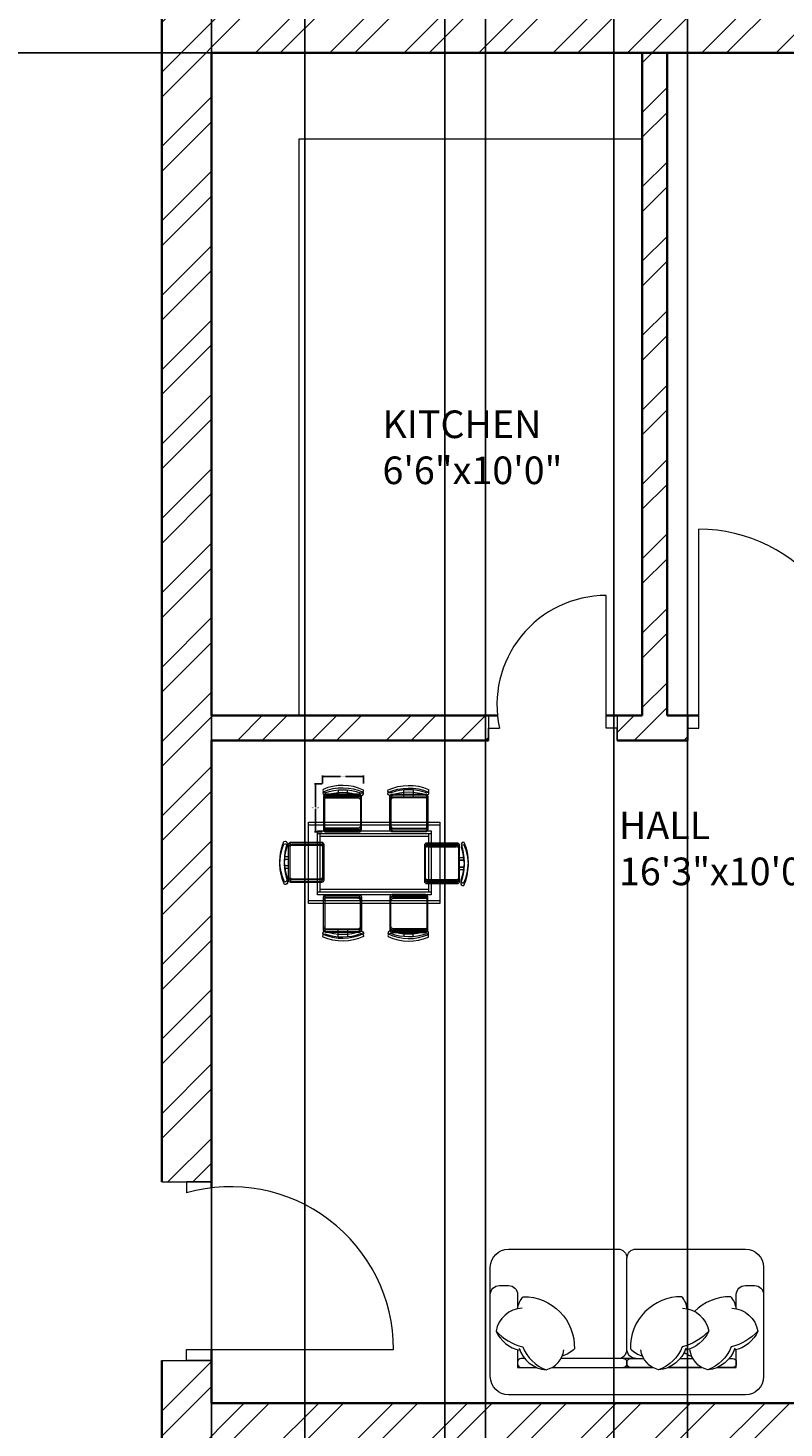
# Model space of a CAD drawing. Units: inches. Extents: x 2552 to 3217, y 1417 to 2737.
# Tile 14 of 25: x 2885 to 3022, y 2138 to 2392. Entities that reach past the tile are written whole.
import ezdxf

# ---------------------------------------------------------------- set-up
doc = ezdxf.new("R2010")
doc.units = ezdxf.units.IN
for name, color, linetype, lineweight in [('A-ANNO-DIMS', 2, 'Continuous', 18), ('A-AREA-IDEN', 7, 'Continuous', 18), ('A-DOOR', 21, 'Continuous', 18), ('A-FLOR-CASE', 9, 'Continuous', 18), ('A-FURN', 8, 'Continuous', 13), ('A-WALL', 7, 'Continuous', 35), ('A-WALL-PATT', 217, 'Continuous', 13)]:
    doc.layers.add(name, color=color, linetype=linetype, lineweight=lineweight)
doc.styles.get("Standard").update_dxf_attribs({"font": 'arial.ttf'})
doc.dimstyles.get("Standard").update_dxf_attribs({"dimtxt": 0.18, "dimasz": 0.18, "dimexe": 0.18, "dimexo": 0.0625, "dimgap": 0.09, "dimtad": 0, "dimtih": 1, "dimtoh": 1, "dimdec": 4, "dimzin": 0, "dimdsep": 46, "dimtxsty": 'Standard', "dimcen": 0.09, "dimadec": 0, "dimazin": 0, "dimtfac": 1, "dimtdec": 4, "dimtofl": 0, "dimtmove": 0, "dimatfit": 3, "dimfxl": 1, "dimtolj": 1, "dimtzin": 0, "dimarcsym": 0})

# ---------------------------------------------------------------- blocks, each defined once
blk = doc.blocks.new('TABLE-DINING-RECT')
for points in [[(0, 14.74), (23.77, 14.74), (23.77, 0.48), (0, 0.48)], [(0, 14.74), (23.77, 14.74), (23.77, 0.48), (0, 0.48)], [(0, 14.26), (23.77, 14.26), (23.77, 0), (0, 0)], [(0, 14.26), (23.77, 14.26), (23.77, 0), (0, 0)], [(1.58, 13.15), (22.19, 13.15), (22.19, 2.06), (1.58, 2.06)], [(1.58, 13.15), (22.19, 13.15), (22.19, 2.06), (1.58, 2.06)], [(1.58, 12.68), (22.19, 12.68), (22.19, 1.59), (1.58, 1.59)], [(1.58, 12.68), (22.19, 12.68), (22.19, 1.58), (1.58, 1.58)], [(2.06, 12.68), (21.71, 12.68), (21.71, 2.54), (2.06, 2.54)], [(2.06, 12.68), (21.71, 12.68), (21.71, 2.54), (2.06, 2.54)], [(2.06, 12.2), (21.71, 12.2), (21.71, 2.06), (2.06, 2.06)], [(2.06, 12.2), (21.71, 12.2), (21.71, 2.06), (2.06, 2.06)]]:
    blk.add_lwpolyline(points, close=True)
blk = doc.blocks.new('DINING-CHAIR-NORTH-WEST')
for points in [[(0.39, 7.1, -0.175809), (6.86, 7.05, 0.578392), (7.35, 7.59, 0.214524), (0.05, 7.69, 0.552014), (0.39, 7.1, -0.065079)], [(0.39, 7.1, -0.175809), (6.86, 7.05, 0.578392), (7.35, 7.59, 0.214524), (0.05, 7.69, 0.552014), (0.39, 7.1, -0.065079)], [(0.39, 6.63, -0.175809), (6.86, 6.58, 0.578392), (7.35, 7.12, 0.214524), (0.05, 7.22, 0.552014), (0.39, 6.63, -0.065079)], [(0.39, 6.63, -0.175809), (6.86, 6.58, 0.578392), (7.35, 7.12, 0.214524), (0.05, 7.22, 0.552014), (0.39, 6.63, -0.065079)], [(6.59, 6.84), (0.58, 6.84, 0.414214), (0.16, 6.42), (0.16, 0.9, 0.414214), (0.58, 0.48), (6.59, 0.48, 0.414214), (7.01, 0.9), (7.01, 6.42, 0.414214), (6.59, 6.84)], [(6.59, 6.84), (0.58, 6.84, 0.414214), (0.16, 6.42), (0.16, 0.9, 0.414214), (0.58, 0.48), (6.59, 0.48, 0.414214), (7.01, 0.9), (7.01, 6.42, 0.414214), (6.59, 6.84)], [(6.59, 6.37), (0.58, 6.37, 0.414214), (0.16, 5.95), (0.16, 0.42, 0.414214), (0.58, 0), (6.59, 0, 0.414214), (7.01, 0.42), (7.01, 5.95, 0.414214), (6.59, 6.37)], [(6.59, 6.37), (0.58, 6.37, 0.414214), (0.16, 5.95), (0.16, 0.42, 0.414214), (0.58, 0), (6.59, 0, 0.414214), (7.01, 0.42), (7.01, 5.95, 0.414214), (6.59, 6.37)], [(4.48, 6.84), (4.48, 7.6, -0.064759)], [(4.48, 6.84), (4.48, 7.6, -0.064759)], [(4.48, 6.37), (4.48, 7.13, -0.064759)], [(4.48, 6.37), (4.48, 7.13, -0.064759)]]:
    blk.add_lwpolyline(points, format="xyb")
for points in [[(2.79, 7.62), (2.79, 6.84)], [(2.79, 7.62), (2.79, 6.84)], [(2.79, 7.14), (2.79, 6.37)], [(2.79, 7.14), (2.79, 6.37)]]:
    blk.add_lwpolyline(points)
for points in [[(0.58, 6.65), (6.4, 6.65, -0.414214), (6.82, 6.23), (6.82, 1.09, -0.414214), (6.4, 0.67), (0.58, 0.67, -0.512069), (0.35, 1.09), (0.35, 6.23, -0.512069)], [(0.58, 6.65), (6.4, 6.65, -0.414214), (6.82, 6.23), (6.82, 1.09, -0.414214), (6.4, 0.67), (0.58, 0.67, -0.512069), (0.35, 1.09), (0.35, 6.23, -0.512069)], [(0.58, 6.18), (6.4, 6.18, -0.414214), (6.82, 5.76), (6.82, 0.61, -0.414214), (6.4, 0.19), (0.58, 0.19, -0.512069), (0.35, 0.61), (0.35, 5.76, -0.512069)], [(0.58, 6.18), (6.4, 6.18, -0.414214), (6.82, 5.76), (6.82, 0.61, -0.414214), (6.4, 0.19), (0.58, 0.19, -0.512069), (0.35, 0.61), (0.35, 5.76, -0.512069)]]:
    blk.add_lwpolyline(points, format="xyb", close=True)
blk = doc.blocks.new('DINING-CHAIR-WEST')
for points in [[(1.37, 0.99, -0.578392), (0.83, 0.5, -0.214524), (0.73, 7.8, -0.552014), (1.32, 7.46, 0.175809), (1.37, 0.99)], [(1.37, 0.99, -0.578392), (0.83, 0.49, -0.214524), (0.73, 7.8, -0.552014), (1.32, 7.46, 0.175809), (1.37, 0.99)], [(1.58, 7.27, -0.414214), (2, 7.69), (7.53, 7.69, -0.414214), (7.95, 7.27), (7.95, 1.26, -0.414214), (7.53, 0.84), (2, 0.84, -0.414214), (1.58, 1.26), (1.58, 7.27)], [(1.58, 7.27, -0.414214), (2, 7.69), (7.53, 7.69, -0.414214), (7.95, 7.27), (7.95, 1.26, -0.414214), (7.53, 0.84), (2, 0.84, -0.414214), (1.58, 1.26), (1.58, 7.27)], [(1.37, 0.51, -0.578392), (0.83, 0.02, -0.214524), (0.73, 7.33, -0.552014), (1.32, 6.98, 0.175809), (1.37, 0.51)], [(1.37, 0.51, -0.578392), (0.83, 0.02, -0.214524), (0.73, 7.33, -0.552014), (1.32, 6.98, 0.175809), (1.37, 0.51)], [(1.58, 6.8, -0.414214), (2, 7.22), (7.53, 7.22, -0.414214), (7.95, 6.8), (7.95, 0.78, -0.414214), (7.53, 0.36), (2, 0.36, -0.414214), (1.58, 0.78), (1.58, 6.8)], [(1.58, 6.8, -0.414214), (2, 7.22), (7.53, 7.22, -0.414214), (7.95, 6.8), (7.95, 0.78, -0.414214), (7.53, 0.36), (2, 0.36, -0.414214), (1.58, 0.78), (1.58, 6.8)], [(1.58, 3.37), (0.82, 3.37, 0.064759)], [(1.58, 3.37), (0.82, 3.37, 0.064759)], [(1.58, 2.9), (0.82, 2.9, 0.064759)], [(1.58, 2.9), (0.82, 2.9, 0.064759)]]:
    blk.add_lwpolyline(points, format="xyb")
for points in [[(1.77, 7.27), (1.77, 1.45, 0.414214), (2.19, 1.03), (7.34, 1.03, 0.414214), (7.76, 1.45), (7.76, 7.27, 0.512069), (7.34, 7.5), (2.19, 7.5, 0.512069)], [(1.77, 7.27), (1.77, 1.45, 0.414214), (2.19, 1.03), (7.34, 1.03, 0.414214), (7.76, 1.45), (7.76, 7.27, 0.512069), (7.34, 7.5), (2.19, 7.5, 0.512069)], [(1.77, 6.79), (1.77, 0.97, 0.414214), (2.19, 0.55), (7.34, 0.55, 0.414214), (7.76, 0.97), (7.76, 6.79, 0.512069), (7.34, 7.03), (2.19, 7.03, 0.512069)], [(1.77, 6.79), (1.77, 0.97, 0.414214), (2.19, 0.55), (7.34, 0.55, 0.414214), (7.76, 0.97), (7.76, 6.79, 0.512069), (7.34, 7.03), (2.19, 7.03, 0.512069)]]:
    blk.add_lwpolyline(points, format="xyb", close=True)
for points in [[(0.81, 5.05), (1.58, 5.05)], [(0.81, 5.05), (1.58, 5.05)], [(0.81, 4.58), (1.58, 4.58)], [(0.81, 4.58), (1.58, 4.58)]]:
    blk.add_lwpolyline(points)
blk = doc.blocks.new('DINING-CHAIR-SOUTH-EAST')
for points in [[(6.8, 2.06, 0.414214), (7.22, 2.48), (7.22, 8.01, 0.414214), (6.8, 8.43), (0.78, 8.43, 0.414214), (0.36, 8.01), (0.36, 2.48, 0.414214), (0.78, 2.06), (6.8, 2.06)], [(6.8, 2.06, 0.414214), (7.22, 2.48), (7.22, 8.01, 0.414214), (6.8, 8.43), (0.78, 8.43, 0.414214), (0.36, 8.01), (0.36, 2.48, 0.414214), (0.78, 2.06), (6.8, 2.06)], [(6.8, 1.58, 0.414214), (7.22, 2), (7.22, 7.53, 0.414214), (6.8, 7.95), (0.78, 7.95, 0.414214), (0.36, 7.53), (0.36, 2, 0.414214), (0.78, 1.58), (6.8, 1.58)], [(6.8, 1.58, 0.414214), (7.22, 2), (7.22, 7.53, 0.414214), (6.8, 7.95), (0.78, 7.95, 0.414214), (0.36, 7.53), (0.36, 2, 0.414214), (0.78, 1.58), (6.8, 1.58)], [(6.98, 1.8, -0.175809), (0.51, 1.85, 0.578392), (0.02, 1.31, 0.214524), (7.33, 1.21, 0.552014), (6.98, 1.8, -0.065079)], [(6.98, 1.8, -0.175809), (0.51, 1.85, 0.578392), (0.02, 1.31, 0.214524), (7.33, 1.21, 0.552014), (6.98, 1.8, -0.065079)], [(6.98, 1.32, -0.175809), (0.51, 1.37, 0.578392), (0.02, 0.83, 0.214524), (7.33, 0.74, 0.552014), (6.98, 1.32, -0.065079)], [(6.98, 1.32, -0.175809), (0.51, 1.37, 0.578392), (0.02, 0.83, 0.214524), (7.33, 0.74, 0.552014), (6.98, 1.32, -0.065079)], [(2.9, 2.06), (2.9, 1.3, -0.064759)], [(2.9, 2.06), (2.9, 1.3, -0.064759)], [(2.9, 1.58), (2.9, 0.82, -0.064759)], [(2.9, 1.58), (2.9, 0.82, -0.064759)]]:
    blk.add_lwpolyline(points, format="xyb")
for points in [[(6.79, 2.25), (0.97, 2.25, -0.414214), (0.55, 2.67), (0.55, 7.82, -0.414214), (0.97, 8.24), (6.79, 8.24, -0.512069), (7.03, 7.82), (7.03, 2.67, -0.512069)], [(6.79, 2.25), (0.97, 2.25, -0.414214), (0.55, 2.67), (0.55, 7.82, -0.414214), (0.97, 8.24), (6.79, 8.24, -0.512069), (7.03, 7.82), (7.03, 2.67, -0.512069)], [(6.79, 1.77), (0.97, 1.77, -0.414214), (0.55, 2.19), (0.55, 7.34, -0.414214), (0.97, 7.76), (6.79, 7.76, -0.512069), (7.03, 7.34), (7.03, 2.19, -0.512069)], [(6.79, 1.77), (0.97, 1.77, -0.414214), (0.55, 2.19), (0.55, 7.34, -0.414214), (0.97, 7.76), (6.79, 7.76, -0.512069), (7.03, 7.34), (7.03, 2.19, -0.512069)]]:
    blk.add_lwpolyline(points, format="xyb", close=True)
for points in [[(4.58, 1.28), (4.58, 2.06)], [(4.58, 1.28), (4.58, 2.06)], [(4.58, 0.81), (4.58, 1.58)], [(4.58, 0.81), (4.58, 1.58)]]:
    blk.add_lwpolyline(points)
blk = doc.blocks.new('*D33')
at = {"layer": 'A-ANNO-DIMS', "color": 0, "lineweight": -2, "transparency": 16777216}
for p, q in [((2937.92, 2254.65), (2936.5, 2254.65)), ((2936.68, 2254.47), (2936.68, 2250.48)), ((2936.68, 2246.13), (2936.68, 2250.11)), ((2937.92, 2245.95), (2936.5, 2245.95))]:
    blk.add_line(p, q, dxfattribs=at)
at = {"layer": 'A-ANNO-DIMS', "color": 0, "transparency": 16777216}
for points in [[(2936.65, 2254.47), (2936.71, 2254.47), (2936.68, 2254.65)], [(2936.65, 2246.13), (2936.71, 2246.13), (2936.68, 2245.95)]]:
    blk.add_solid(points, dxfattribs=at)
at = {"layer": 'Defpoints', "color": 0, "transparency": 16777216}
for p in [(2936.68, 2254.65), (2937.98, 2254.65), (2937.98, 2245.95)]:
    blk.add_point(p, dxfattribs=at)
at = {"layer": 'A-ANNO-DIMS', "color": 0, "transparency": 16777216, "insert": (2936.68, 2250.3), "char_height": 0.18, "attachment_point": 5}
blk.add_mtext('\\A1;CHAIR 9 TYP.', dxfattribs=at)
blk = doc.blocks.new('*D34')
at = {"layer": 'A-ANNO-DIMS', "color": 0, "lineweight": -2, "transparency": 16777216}
for p, q in [((2937.98, 2254.71), (2937.98, 2256.14)), ((2938.16, 2255.96), (2941.24, 2255.96)), ((2945.22, 2255.96), (2942.15, 2255.96)), ((2945.4, 2254.71), (2945.4, 2256.14))]:
    blk.add_line(p, q, dxfattribs=at)
at = {"layer": 'A-ANNO-DIMS', "color": 0, "transparency": 16777216}
for points in [[(2938.16, 2255.99), (2938.16, 2255.93), (2937.98, 2255.96)], [(2945.22, 2255.99), (2945.22, 2255.93), (2945.4, 2255.96)]]:
    blk.add_solid(points, dxfattribs=at)
at = {"layer": 'Defpoints', "color": 0, "transparency": 16777216}
for p in [(2937.98, 2254.65), (2945.4, 2255.96), (2945.4, 2254.65)]:
    blk.add_point(p, dxfattribs=at)
at = {"layer": 'A-ANNO-DIMS', "color": 0, "transparency": 16777216, "insert": (2941.69, 2255.96), "char_height": 0.18, "attachment_point": 5}
blk.add_mtext('\\A1;7 TYP.', dxfattribs=at)
blk = doc.blocks.new('*D56')
at = {"layer": 'A-ANNO-DIMS', "color": 0, "lineweight": -2, "transparency": 16777216}
for p, q in [((2967.49, 2515.95), (2967.49, 1482.53)), ((2990.69, 2515.95), (2990.69, 1482.53)), ((2967.67, 1482.71), (2978.76, 1482.71)), ((2990.51, 1482.71), (2979.41, 1482.71))]:
    blk.add_line(p, q, dxfattribs=at)
at = {"layer": 'A-ANNO-DIMS', "color": 0, "transparency": 16777216}
for points in [[(2967.67, 1482.74), (2967.67, 1482.68), (2967.49, 1482.71)], [(2990.51, 1482.74), (2990.51, 1482.68), (2990.69, 1482.71)]]:
    blk.add_solid(points, dxfattribs=at)
at = {"layer": 'Defpoints', "color": 0, "transparency": 16777216}
for p in [(2967.49, 2516.01), (2990.69, 2516.01), (2990.69, 1482.71)]:
    blk.add_point(p, dxfattribs=at)
at = {"layer": 'A-ANNO-DIMS', "color": 0, "transparency": 16777216, "insert": (2979.09, 1482.71), "char_height": 0.18, "attachment_point": 5}
blk.add_mtext('\\A1;23.2', dxfattribs=at)
blk = doc.blocks.new('*D57')
at = {"layer": 'A-ANNO-DIMS', "color": 0, "lineweight": -2, "transparency": 16777216}
for p, q in [((3004.08, 2515.95), (3004.08, 1482.53)), ((3036.34, 2515.95), (3036.34, 1482.53)), ((3004.26, 1482.71), (3019.75, 1482.71)), ((3036.16, 1482.71), (3020.68, 1482.71))]:
    blk.add_line(p, q, dxfattribs=at)
at = {"layer": 'A-ANNO-DIMS', "color": 0, "transparency": 16777216}
for points in [[(3004.26, 1482.74), (3004.26, 1482.68), (3004.08, 1482.71)], [(3036.16, 1482.74), (3036.16, 1482.68), (3036.34, 1482.71)]]:
    blk.add_solid(points, dxfattribs=at)
at = {"layer": 'Defpoints', "color": 0, "transparency": 16777216}
for p in [(3004.08, 2516.01), (3036.34, 2516.01), (3036.34, 1482.71)]:
    blk.add_point(p, dxfattribs=at)
at = {"layer": 'A-ANNO-DIMS', "color": 0, "transparency": 16777216, "insert": (3020.21, 1482.71), "char_height": 0.18, "attachment_point": 5}
blk.add_mtext('\\A1;32.255', dxfattribs=at)
blk = doc.blocks.new('*D64')
at = {"layer": 'A-ANNO-DIMS', "color": 0, "lineweight": -2, "transparency": 16777216}
for p, q in [((2646.35, 1551.58), (2646.35, 2709.49)), ((2646.53, 2709.31), (2802.77, 2709.31)), ((2959.93, 2709.31), (2803.69, 2709.31)), ((2960.11, 1551.58), (2960.11, 2709.49))]:
    blk.add_line(p, q, dxfattribs=at)
at = {"layer": 'A-ANNO-DIMS', "color": 0, "transparency": 16777216}
for points in [[(2646.53, 2709.34), (2646.53, 2709.28), (2646.35, 2709.31)], [(2959.93, 2709.34), (2959.93, 2709.28), (2960.11, 2709.31)]]:
    blk.add_solid(points, dxfattribs=at)
at = {"layer": 'Defpoints', "color": 0, "transparency": 16777216}
for p in [(2960.11, 2709.31), (2646.35, 1551.51), (2960.11, 1551.51)]:
    blk.add_point(p, dxfattribs=at)
at = {"layer": 'A-ANNO-DIMS', "color": 0, "transparency": 16777216, "insert": (2803.23, 2709.31), "char_height": 0.18, "attachment_point": 5}
blk.add_mtext('\\A1;313.76', dxfattribs=at)
blk = doc.blocks.new('*D67')
at = {"layer": 'A-ANNO-DIMS', "color": 0, "lineweight": -2, "transparency": 16777216}
for p, q in [((2917.85, 2640.45), (2917.85, 1482.53)), ((2934.77, 2624.73), (2934.77, 1482.53)), ((2918.03, 1482.71), (2925.86, 1482.71)), ((2934.59, 1482.71), (2926.76, 1482.71))]:
    blk.add_line(p, q, dxfattribs=at)
at = {"layer": 'A-ANNO-DIMS', "color": 0, "transparency": 16777216}
for points in [[(2918.03, 1482.74), (2918.03, 1482.68), (2917.85, 1482.71)], [(2934.59, 1482.74), (2934.59, 1482.68), (2934.77, 1482.71)]]:
    blk.add_solid(points, dxfattribs=at)
at = {"layer": 'Defpoints', "color": 0, "transparency": 16777216}
for p in [(2917.85, 2640.51), (2934.77, 2624.79), (2934.77, 1482.71)]:
    blk.add_point(p, dxfattribs=at)
at = {"layer": 'A-ANNO-DIMS', "color": 0, "transparency": 16777216, "insert": (2926.31, 1482.71), "char_height": 0.18, "attachment_point": 5}
blk.add_mtext('\\A1;16.912', dxfattribs=at)
blk = doc.blocks.new('*D69')
at = {"layer": 'A-ANNO-DIMS', "color": 0, "lineweight": -2, "transparency": 16777216}
for p, q in [((2908.79, 2403.41), (2577.37, 2403.41)), ((2577.55, 2403.23), (2577.55, 2395.39)), ((2577.55, 2387.19), (2577.55, 2395.03)), ((2917.79, 2387.01), (2577.37, 2387.01))]:
    blk.add_line(p, q, dxfattribs=at)
at = {"layer": 'A-ANNO-DIMS', "color": 0, "transparency": 16777216}
for points in [[(2577.52, 2403.23), (2577.58, 2403.23), (2577.55, 2403.41)], [(2577.52, 2387.19), (2577.58, 2387.19), (2577.55, 2387.01)]]:
    blk.add_solid(points, dxfattribs=at)
at = {"layer": 'Defpoints', "color": 0, "transparency": 16777216}
for p in [(2577.55, 2403.41), (2908.85, 2403.41), (2917.85, 2387.01)]:
    blk.add_point(p, dxfattribs=at)
at = {"layer": 'A-ANNO-DIMS', "color": 0, "transparency": 16777216, "insert": (2577.55, 2395.21), "char_height": 0.18, "attachment_point": 5}
blk.add_mtext('\\A1;16.4', dxfattribs=at)

msp = doc.modelspace()

# ---------------------------------------------------------------- hatches: boundary and pattern name
at = {"layer": 'A-WALL-PATT'}
h = msp.add_hatch(dxfattribs=at)
h.set_pattern_fill('ANSI32', color=256)
h.paths.add_polyline_path([(2756.676, 2649.5125), (2637.3535, 2649.5125), (2637.3535, 2617.9626), (2641.8535, 2617.9626), (2646.3535, 2617.9626), (2646.3535, 2640.5125), (2724.3535, 2640.5125), (2724.3535, 2520.5125), (2720.299, 2520.5125), (2720.299, 2516.0125), (2733.4075, 2516.0125), (2733.4075, 2518.2213), (2733.4075, 2520.5125), (2728.8535, 2520.5125), (2728.8535, 2640.5125), (2756.676, 2640.5125)])
h.paths.add_polyline_path([(2848.8535, 2649.5125), (2804.676, 2649.5125), (2804.676, 2640.5125), (2839.8535, 2640.5125), (2839.8535, 2598.3517), (2848.8535, 2598.3517)])
h.paths.add_polyline_path([(2646.3535, 2516.0125), (2697.9593, 2516.0125), (2697.9593, 2518.2625), (2697.9593, 2520.5125), (2646.3535, 2520.5125), (2646.3535, 2581.9626), (2637.3535, 2581.9626), (2637.3535, 2364.3298), (2646.3535, 2364.3298), (2646.3535, 2387.0125), (2724.3535, 2387.0125), (2724.3535, 2267.0125), (2721.0443, 2267.0125), (2721.0443, 2262.5125), (2733.7854, 2262.5125), (2733.7854, 2264.7625), (2733.7854, 2267.0125), (2728.8535, 2267.0125), (2728.8535, 2387.0125), (2839.8535, 2387.0125), (2839.8535, 2363.8387), (2848.8535, 2363.8387), (2848.8535, 2403.7415), (2844.3535, 2403.7415), (2839.8535, 2403.7415), (2839.8535, 2396.0125), (2646.3535, 2396.0125)])
h.paths.add_polyline_path([(2848.8535, 2550.3517), (2844.3535, 2550.3517), (2839.8535, 2550.3517), (2839.8535, 2520.5125), (2801.9195, 2520.5125), (2801.9195, 2518.2625), (2801.9195, 2516.0125), (2839.8535, 2516.0125), (2839.8535, 2507.5813), (2848.8535, 2507.5813)], flags=17)
h.paths.add_polyline_path([(2848.8535, 2483.5813), (2844.3535, 2483.5813), (2839.8535, 2483.5813), (2839.8535, 2468.0125), (2773.8535, 2468.0125), (2773.8535, 2516.0125), (2778.1336, 2516.0125), (2778.1336, 2520.5125), (2766.696, 2520.5125), (2766.696, 2518.2625), (2766.696, 2516.0125), (2769.3535, 2516.0125), (2769.3535, 2463.5125), (2839.8535, 2463.5125), (2839.8535, 2431.0782), (2848.8535, 2431.0782)], flags=17)
h.paths.add_polyline_path([(2917.8535, 2569.2764), (2913.3535, 2569.2764), (2908.8535, 2569.2764), (2908.8535, 2433.001), (2917.8535, 2433.001), (2917.8535, 2516.0125), (2967.486, 2516.0125), (2967.486, 2520.5125), (2917.8535, 2520.5125)])
h.paths.add_polyline_path([(3000.3535, 2640.5125), (2995.8535, 2640.5125), (2995.8535, 2520.5125), (2990.688, 2520.5125), (2990.688, 2516.0125), (3004.0844, 2516.0125), (3004.0844, 2518.2625), (3004.0844, 2520.5125), (3000.3535, 2520.5125)])
h.paths.add_polyline_path([(3120.3535, 2561.3689), (3115.8535, 2561.3689), (3111.3535, 2561.3689), (3111.3535, 2520.5125), (3070.9814, 2520.5125), (3070.9814, 2518.2625), (3070.9814, 2516.0125), (3111.3535, 2516.0125), (3111.3535, 2505.1841), (3120.3535, 2505.1841)])
h.paths.add_polyline_path([(3120.3535, 2481.1841), (3115.8535, 2481.1841), (3111.3535, 2481.1841), (3111.3535, 2468.0125), (3045.3535, 2468.0125), (3045.3535, 2516.0125), (3048.9787, 2516.0125), (3048.9787, 2520.5125), (3036.3395, 2520.5125), (3036.3395, 2516.0125), (3040.8535, 2516.0125), (3040.8535, 2463.5125), (3111.3535, 2463.5125), (3111.3535, 2396.0125), (2917.8535, 2396.0125), (2917.8535, 2403.4124), (2913.3535, 2403.4124), (2908.8535, 2403.4124), (2908.8535, 2182.5756), (2917.8535, 2182.5756), (2917.8535, 2262.5125), (2968.001, 2262.5125), (2968.001, 2264.7625), (2968.001, 2267.0125), (2917.8535, 2267.0125), (2917.8535, 2387.0125), (3111.3535, 2387.0125), (3111.3535, 2352.2435), (3120.3535, 2352.2435)])
h.paths.add_polyline_path([(3120.3535, 2304.2435), (3115.8535, 2304.2435), (3111.3535, 2304.2435), (3111.3535, 2267.0125), (3073.8616, 2267.0125), (3073.8616, 2264.7625), (3073.8616, 2262.5125), (3111.3535, 2262.5125), (3111.3535, 2252.376), (3120.3535, 2252.376)], flags=17)
h.paths.add_polyline_path([(3120.3535, 2228.376), (3115.8535, 2228.376), (3111.3535, 2228.376), (3111.3535, 2214.5125), (3045.3535, 2214.5125), (3045.3535, 2262.5125), (3049.3096, 2262.5125), (3049.3096, 2267.0125), (3035.0125, 2267.0125), (3035.0125, 2262.5125), (3040.8535, 2262.5125), (3040.8535, 2210.0125), (3111.3535, 2210.0125), (3111.3535, 2142.5125), (2917.8535, 2142.5125), (2917.8535, 2150.2408), (2913.3535, 2150.2408), (2908.8535, 2150.2408), (2908.8535, 1924.9905), (2917.8535, 1924.9905), (2917.8535, 2009.0125), (2971.959, 2009.0125), (2971.959, 2011.2625), (2971.959, 2013.5125), (2917.8535, 2013.5125), (2917.8535, 2133.5125), (2995.8535, 2133.5125), (2995.8535, 2013.5125), (2992.1797, 2013.5125), (2992.1797, 2009.0125), (3004.3344, 2009.0125), (3004.3344, 2011.2625), (3004.3344, 2013.5125), (3000.3535, 2013.5125), (3000.3535, 2133.5125), (3111.3535, 2133.5125), (3111.3535, 2115.0291), (3120.3535, 2115.0291)])
h.paths.add_polyline_path([(3000.3535, 2387.0125), (2995.8535, 2387.0125), (2995.8535, 2267.0125), (2991.3326, 2267.0125), (2991.3326, 2262.5125), (3004.1044, 2262.5125), (3004.1044, 2264.7625), (3004.1044, 2267.0125), (3000.3535, 2267.0125)], flags=17)
h.paths.add_polyline_path([(3120.3535, 1973.2388), (3115.8535, 1973.2388), (3111.3535, 1973.2388), (3111.3535, 1961.0125), (3045.3535, 1961.0125), (3045.3535, 2009.0125), (3048.9101, 2009.0125), (3048.9101, 2013.5125), (3037.105, 2013.5125), (3037.105, 2011.2625), (3037.105, 2009.0125), (3040.8535, 2009.0125), (3040.8535, 1956.5125), (3111.3535, 1956.5125), (3111.3535, 1889.0125), (2917.8535, 1889.0125), (2917.8535, 1895.7215), (2913.3535, 1895.7215), (2908.8535, 1895.7215), (2908.8535, 1844.2217), (2917.8535, 1844.2217), (2917.8535, 1880.0125), (3111.3535, 1880.0125), (3111.3535, 1846.9541), (3120.3535, 1846.9541)])
h.paths.add_polyline_path([(3120.3535, 2067.0291), (3111.3535, 2067.0291), (3111.3535, 2013.5125), (3071.3001, 2013.5125), (3071.3001, 2009.0125), (3111.3535, 2009.0125), (3111.3535, 1997.2388), (3120.3535, 1997.2388)], flags=0)
h.paths.add_polyline_path([(3120.3535, 1798.9541), (3115.8535, 1798.9541), (3111.3535, 1798.9541), (3111.3535, 1760.0125), (3071.2497, 1760.0125), (3071.2497, 1757.7625), (3071.2497, 1755.5125), (3111.3535, 1755.5125), (3111.3535, 1746.162), (3120.3535, 1746.2478)])
h.paths.add_polyline_path([(3120.3535, 1722.2049), (3111.3535, 1722.2049), (3111.3535, 1707.5125), (3045.3535, 1707.5125), (3045.3535, 1755.5125), (3048.6624, 1755.5125), (3048.6624, 1760.0125), (3035.3703, 1760.0125), (3035.3703, 1755.5125), (3040.8535, 1755.5125), (3040.8535, 1703.0125), (3111.3535, 1703.0125), (3111.3535, 1635.5125), (2917.8535, 1635.5125), (2917.8535, 1643.1366), (2913.3535, 1643.1366), (2908.8535, 1643.1366), (2908.8535, 1626.5125), (3120.3535, 1626.5125)])
h.paths.add_polyline_path([(2917.8535, 1755.5125), (2973.2287, 1755.5125), (2973.2287, 1757.7625), (2973.2287, 1760.0125), (2917.8535, 1760.0125), (2917.8535, 1808.2217), (2913.3535, 1808.2217), (2908.8535, 1808.2217), (2908.8535, 1676.1665), (2917.8535, 1676.1665)])
h.paths.add_polyline_path([(3000.3535, 1880.0125), (2995.8535, 1880.0125), (2995.8535, 1760.0125), (2992.9329, 1760.0125), (2992.9329, 1755.5125), (3003.8766, 1755.5125), (3003.8766, 1757.7625), (3003.8766, 1760.0125), (3000.3535, 1760.0125)])
h.paths.add_polyline_path([(2848.8535, 1896.6971), (2844.3535, 1896.6971), (2839.8535, 1896.6971), (2839.8535, 1889.0125), (2646.3535, 1889.0125), (2646.3535, 2009.0125), (2700.5253, 2009.0125), (2700.5253, 2011.2625), (2700.5253, 2013.5125), (2646.3535, 2013.5125), (2646.3535, 2053.1812), (2641.8535, 2053.1812), (2637.3535, 2053.1812), (2637.3535, 1836.254), (2646.3535, 1836.254), (2646.3535, 1880.0125), (2724.3535, 1880.0125), (2724.3535, 1760.0125), (2721.2473, 1760.0125), (2721.2473, 1755.5125), (2731.9187, 1755.5125), (2731.9187, 1757.7625), (2731.9187, 1760.0125), (2728.8535, 1760.0125), (2728.8535, 1880.0125), (2839.8535, 1880.0125), (2839.8535, 1840.3813), (2848.8535, 1840.3813)])
h.paths.add_polyline_path([(2848.8535, 1792.3813), (2844.3535, 1792.3813), (2839.8535, 1792.3813), (2839.8535, 1760.0125), (2797.8845, 1760.0125), (2797.8845, 1755.5125), (2839.8535, 1755.5125), (2839.8535, 1743.3688), (2844.3535, 1743.3688), (2848.8535, 1743.3688)], flags=0)
h.paths.add_polyline_path([(2848.8535, 1719.3688), (2844.3535, 1719.3688), (2839.8535, 1719.3688), (2839.8535, 1707.5125), (2773.8535, 1707.5125), (2773.8535, 1755.5125), (2777.716, 1755.5125), (2777.716, 1760.0125), (2760.9247, 1760.0125), (2760.9247, 1757.9721), (2760.9247, 1755.5125), (2769.3535, 1755.5125), (2769.3535, 1703.0125), (2839.8535, 1703.0125), (2839.8535, 1673.0277), (2848.8535, 1672.9407)], flags=0)
h.paths.add_polyline_path([(2646.3535, 1755.5125), (2702.9171, 1755.5125), (2702.9171, 1757.7625), (2702.9171, 1760.0125), (2646.3535, 1760.0125), (2646.3535, 1800.254), (2641.8535, 1800.254), (2637.3535, 1800.254), (2637.3535, 1626.5125), (2848.8535, 1626.5125), (2848.8535, 1643.1187), (2844.3535, 1643.1187), (2839.8535, 1643.1187), (2839.8535, 1635.5125), (2646.3535, 1635.5125)])
h.paths.add_polyline_path([(2848.8535, 2148.8427), (2844.3535, 2148.8427), (2839.8535, 2148.8427), (2839.8535, 2142.5125), (2646.3535, 2142.5125), (2646.3535, 2262.5125), (2701.3562, 2262.5125), (2701.3562, 2264.7625), (2701.3562, 2267.0125), (2646.3535, 2267.0125), (2646.3535, 2328.3298), (2637.3535, 2328.3298), (2637.3535, 2089.1812), (2646.3535, 2089.1812), (2646.3535, 2133.5125), (2839.8535, 2133.5125), (2839.8535, 2097.5966), (2848.8535, 2097.5966)])
h.paths.add_polyline_path([(2728.8535, 2133.5125), (2724.3535, 2133.5125), (2724.3535, 2013.5125), (2719.6039, 2013.5125), (2719.6039, 2009.0125), (2732.5784, 2009.0125), (2732.5784, 2011.2625), (2732.5784, 2013.5125), (2728.8535, 2013.5125)])
h.paths.add_polyline_path([(2848.8535, 1970.0557), (2844.3535, 1970.0557), (2839.8535, 1970.0557), (2839.8535, 1961.0125), (2773.8535, 1961.0125), (2773.8535, 2009.0125), (2777.3388, 2009.0125), (2777.3388, 2013.5125), (2764.7681, 2013.5125), (2764.7681, 2009.0125), (2769.3535, 2009.0125), (2769.3535, 1956.5125), (2839.8535, 1956.5125), (2839.8535, 1924.7199), (2848.8535, 1924.7199)], flags=17)
h.paths.add_polyline_path([(2848.8535, 2049.5966), (2844.3535, 2049.5966), (2839.8535, 2049.5966), (2839.8535, 2013.5125), (2798.198, 2013.5125), (2798.198, 2011.2625), (2798.198, 2009.0125), (2839.8535, 2009.0125), (2839.8535, 1994.0557), (2848.8535, 1994.0557)], flags=17)
h.paths.add_polyline_path([(2848.8535, 2315.8387), (2839.8535, 2315.8387), (2839.8535, 2267.0125), (2799.3375, 2267.0125), (2799.3375, 2264.7625), (2799.3375, 2262.5125), (2839.8535, 2262.5125), (2839.8535, 2253.2843), (2848.8535, 2253.2843)], flags=17)
h.paths.add_polyline_path([(2848.8535, 2229.2843), (2839.8535, 2229.2843), (2839.8535, 2177.6936), (2848.8535, 2177.6936)], flags=17)
h.paths.add_polyline_path([(2839.8535, 2214.5125), (2773.8535, 2214.5125), (2773.8535, 2262.5125), (2777.6984, 2262.5125), (2777.6984, 2267.0125), (2763.8226, 2267.0125), (2763.8226, 2262.5125), (2769.3535, 2262.5125), (2769.3535, 2210.0125), (2839.8535, 2210.0125)], flags=17)
h.paths.add_polyline_path([(3050.32, 2520.2817), (3088.9114, 2520.2817), (3088.9114, 2538.939), (3050.32, 2538.939)], flags=9)

# ---------------------------------------------------------------- linework, layer by layer
at = {"layer": 'A-DOOR'}
for p, q in [((3006.1044, 2264.7625), (3006.1044, 2300.7625)), ((2989.3326, 2264.7625), (2989.3326, 2288.7625)), ((2968.001, 2267.0125), (2968.001, 2262.5125)), ((2991.3326, 2267.0125), (2991.3326, 2262.5125)), ((3004.1044, 2267.0125), (3004.1044, 2262.5125)), ((2968.001, 2262.5125), (2968.001, 2264.7625)), ((2968.001, 2264.7625), (2970.001, 2264.7625)), ((2991.3326, 2264.7625), (2989.3326, 2264.7625)), ((2991.3326, 2262.5125), (2991.3326, 2264.7625)), ((3004.1044, 2262.5125), (3004.1044, 2264.7625)), ((3004.1044, 2264.7625), (3006.1044, 2264.7625)), ((2908.8535, 2182.5756), (2917.8535, 2182.5756)), ((2917.8535, 2182.5756), (2913.3535, 2182.5756)), ((2913.3535, 2182.5756), (2913.3535, 2180.5756)), ((2913.3535, 2150.2408), (2913.3535, 2152.2408)), ((2913.3535, 2152.2408), (2950.81, 2152.2408)), ((2908.8535, 2150.2408), (2917.8535, 2150.2408)), ((2917.8535, 2150.2408), (2913.3535, 2150.2408))]:
    msp.add_line(p, q, dxfattribs=at)
for centre, radius, start, end in [((3006.1044, 2272.7064), 28.0562, 343.552291, 90), ((2989.3326, 2268.9768), 19.7857, 90, 192.298057), ((2921.3645, 2152.2408), 29.4455, 0, 105.787056)]:
    msp.add_arc(centre, radius, start, end, dxfattribs=at)
at = {"layer": 'A-FLOR-CASE'}
for p, q in [((2933.7382, 2267.0125), (2933.7382, 2371.4144)), ((2933.7382, 2371.4144), (2995.8535, 2371.4144))]:
    msp.add_line(p, q, dxfattribs=at)
at = {"layer": 'A-FURN'}
for points in [[(2950.3169, 2252.9994, -0.57839206), (2949.8264, 2253.5388, -0.21452438), (2957.1347, 2253.6368, -0.55201397), (2956.7913, 2253.0485, 0.1758092), (2950.3169, 2252.9994)], [(2950.3169, 2252.524, -0.57839206), (2949.8264, 2253.0634, -0.21452438), (2957.1347, 2253.1614, -0.55201397), (2956.7913, 2252.5731, 0.1758092), (2950.3169, 2252.524)], [(2950.3169, 2252.9992, -0.57839206), (2949.8264, 2253.5385, -0.21452438), (2957.1347, 2253.6366, -0.55201397), (2956.7913, 2253.0482, 0.1758092), (2950.3169, 2252.9992)], [(2950.3169, 2252.5238, -0.57839206), (2949.8264, 2253.0631, -0.21452438), (2957.1347, 2253.1612, -0.55201397), (2956.7913, 2252.5728, 0.1758092), (2950.3169, 2252.5238)], [(2956.6022, 2252.7886, -0.41421356), (2957.0227, 2252.3681), (2957.0227, 2246.8414, -0.41421356), (2956.6022, 2246.4209), (2950.5916, 2246.4209, -0.41421356), (2950.171, 2246.8414), (2950.171, 2252.3681, -0.41421356), (2950.5916, 2252.7886), (2956.6022, 2252.7886)], [(2956.6022, 2252.3132, -0.41421356), (2957.0227, 2251.8927), (2957.0227, 2246.366, -0.41421356), (2956.6022, 2245.9455), (2950.5916, 2245.9455, -0.41421356), (2950.171, 2246.366), (2950.171, 2251.8927, -0.41421356), (2950.5916, 2252.3132), (2956.6022, 2252.3132)], [(2956.6022, 2252.7884, -0.41421356), (2957.0227, 2252.3678), (2957.0227, 2246.8412, -0.41421356), (2956.6022, 2246.4206), (2950.5916, 2246.4206, -0.41421356), (2950.1711, 2246.8412), (2950.1711, 2252.3678, -0.41421356), (2950.5916, 2252.7884), (2956.6022, 2252.7884)], [(2956.6022, 2252.3129, -0.41421356), (2957.0227, 2251.8924), (2957.0227, 2246.3657, -0.41421356), (2956.6022, 2245.9452), (2950.5916, 2245.9452, -0.41421356), (2950.1711, 2246.3657), (2950.1711, 2251.8924, -0.41421356), (2950.5916, 2252.3129), (2956.6022, 2252.3129)], [(2952.7028, 2252.7886), (2952.7028, 2253.5488, 0.06475861)], [(2952.7028, 2252.7884), (2952.7028, 2253.5485, 0.06475861)], [(2952.7028, 2252.3132), (2952.7028, 2253.0734, 0.06475861)], [(2952.7028, 2252.3129), (2952.7028, 2253.0731, 0.06475861)], [(2962.7812, 2243.4931, 0.41421356), (2962.3607, 2243.9137), (2956.834, 2243.9137, 0.41421356), (2956.4135, 2243.4931), (2956.4135, 2237.4825, 0.41421356), (2956.834, 2237.062), (2962.3607, 2237.062, 0.41421356), (2962.7812, 2237.4825), (2962.7812, 2243.4931)], [(2962.7812, 2243.4929, 0.41421356), (2962.3607, 2243.9134), (2956.834, 2243.9134, 0.41421356), (2956.4135, 2243.4929), (2956.4135, 2237.4822, 0.41421356), (2956.834, 2237.0617), (2962.3607, 2237.0617, 0.41421356), (2962.7812, 2237.4822), (2962.7812, 2243.4929)], [(2963.041, 2243.6822, -0.17580919), (2962.992, 2237.2078, 0.57839206), (2963.5313, 2236.7173, 0.21452438), (2963.6294, 2244.0256, 0.55201397), (2963.041, 2243.6822, -0.06507904)], [(2963.041, 2243.682, -0.17580919), (2962.992, 2237.2075, 0.57839206), (2963.5313, 2236.7171, 0.21452438), (2963.6294, 2244.0253, 0.55201397), (2963.041, 2243.682, -0.06507904)], [(2963.041, 2243.2068, -0.17580919), (2962.992, 2236.7324, 0.57839206), (2963.5313, 2236.2419, 0.21452438), (2963.6294, 2243.5502, 0.55201397), (2963.041, 2243.2068, -0.06507904)], [(2963.041, 2243.2066, -0.17580919), (2962.992, 2236.7321, 0.57839206), (2963.5313, 2236.2416, 0.21452438), (2963.6294, 2243.5499, 0.55201397), (2963.041, 2243.2066, -0.06507904)], [(2962.7812, 2243.0177, 0.41421356), (2962.3607, 2243.4382), (2956.834, 2243.4382, 0.41421356), (2956.4135, 2243.0177), (2956.4135, 2237.0071, 0.41421356), (2956.834, 2236.5866), (2962.3607, 2236.5866, 0.41421356), (2962.7812, 2237.0071), (2962.7812, 2243.0177)], [(2962.7812, 2243.0175, 0.41421356), (2962.3607, 2243.438), (2956.834, 2243.438, 0.41421356), (2956.4135, 2243.0175), (2956.4135, 2237.0068, 0.41421356), (2956.834, 2236.5863), (2962.3607, 2236.5863, 0.41421356), (2962.7812, 2237.0068), (2962.7812, 2243.0175)], [(2962.7812, 2239.5937), (2963.5413, 2239.5937, -0.06475861)], [(2962.7812, 2239.5935), (2963.5414, 2239.5935, -0.06475861)], [(2962.7812, 2239.1183), (2963.5413, 2239.1183, -0.06475861)], [(2962.7812, 2239.1181), (2963.5414, 2239.1181, -0.06475861)], [(2944.5915, 2228.2211), (2938.5809, 2228.2211, -0.41421356), (2938.1604, 2228.6416), (2938.1604, 2234.1683, -0.41421356), (2938.5809, 2234.5888), (2944.5915, 2234.5888, -0.41421356), (2945.0121, 2234.1683), (2945.0121, 2228.6416, -0.41421356), (2944.5915, 2228.2211)], [(2944.5916, 2228.2209), (2938.5809, 2228.2209, -0.41421356), (2938.1604, 2228.6414), (2938.1604, 2234.1681, -0.41421356), (2938.5809, 2234.5886), (2944.5916, 2234.5886, -0.41421356), (2945.0121, 2234.1681), (2945.0121, 2228.6414, -0.41421356), (2944.5916, 2228.2209)], [(2944.5915, 2227.7457), (2938.5809, 2227.7457, -0.41421356), (2938.1604, 2228.1662), (2938.1604, 2233.6929, -0.41421356), (2938.5809, 2234.1134), (2944.5915, 2234.1134, -0.41421356), (2945.0121, 2233.6929), (2945.0121, 2228.1662, -0.41421356), (2944.5915, 2227.7457)], [(2944.5916, 2227.7455), (2938.5809, 2227.7455, -0.41421356), (2938.1604, 2228.166), (2938.1604, 2233.6927, -0.41421356), (2938.5809, 2234.1132), (2944.5916, 2234.1132, -0.41421356), (2945.0121, 2233.6927), (2945.0121, 2228.166, -0.41421356), (2944.5916, 2227.7455)], [(2944.8662, 2228.0103, -0.57839206), (2945.3567, 2227.471, -0.21452438), (2938.0484, 2227.3729, -0.55201397), (2938.3918, 2227.9613, 0.17580929), (2944.8662, 2228.0103)], [(2944.8662, 2227.5349, -0.57839206), (2945.3567, 2226.9956, -0.21452438), (2938.0484, 2226.8975, -0.55201397), (2938.3918, 2227.4859, 0.17580929), (2944.8662, 2227.5349)], [(2944.8662, 2228.0101, -0.57839206), (2945.3567, 2227.4707, -0.21452438), (2938.0484, 2227.3727, -0.55201397), (2938.3918, 2227.961, 0.17580929), (2944.8662, 2228.0101)], [(2944.8662, 2227.5346, -0.57839206), (2945.3567, 2226.9953, -0.21452438), (2938.0484, 2226.8973, -0.55201397), (2938.3918, 2227.4856, 0.17580929), (2944.8662, 2227.5346)], [(2942.4803, 2228.2211), (2942.4803, 2227.461, 0.06475861)], [(2942.4803, 2228.2209), (2942.4803, 2227.4607, 0.06475861)], [(2942.4803, 2227.7457), (2942.4803, 2226.9856, 0.06475861)], [(2942.4803, 2227.7455), (2942.4803, 2226.9853, 0.06475861)], [(2991.4414, 2150.6144, 0.41421356), (2993.091, 2152.264), (2993.091, 2168.7596, 0.41421356)], [(2994.7406, 2150.6144, -0.41421356), (2993.091, 2152.264), (2993.091, 2168.7596, -0.41421356)], [(2968.3475, 2162.1613, -0.41421356), (2969.9971, 2163.8109), (2971.6467, 2163.8109, -0.41421356), (2973.2962, 2162.1613), (2973.2962, 2159.6056)], [(3012.8858, 2159.6056), (3012.8858, 2162.1613, -0.41421356), (3014.5353, 2163.8109), (3016.1849, 2163.8109, -0.41421356), (3017.8344, 2162.1613)], [(2973.2926, 2159.6048, -0.16554063), (2974.3131, 2161.7844, -0.42598917), (2983.5774, 2152.3345, -0.12152332), (2981.3782, 2151.0321, 7.11546429)], [(3004.0032, 2159.6048, 0.16554063), (3002.9827, 2161.7844, 0.42598917), (2993.7185, 2152.3345, 0.12152332), (2995.9176, 2151.0321, -7.11546429)], [(3012.8893, 2159.6048, 0.16554063), (3011.8689, 2161.7844, 0.20023115), (3005.3207, 2159.1299, 0.12152332)], [(2974.1241, 2159.7054, 0.35677236), (2969.3974, 2155.5475, 0.24954205), (2973.6802, 2152.121, -9.61688035)], [(3003.1718, 2159.7054, -0.35677236), (3007.8985, 2155.5475, -0.24954205), (3003.6157, 2152.121, 9.61688035)], [(3012.0579, 2159.7054, -0.35677236), (3016.7846, 2155.5475, -0.24954205), (3012.5018, 2152.121, 9.61688035)], [(2969.3974, 2155.5475, 0.14772988), (2974.2186, 2152.7125, 0.21334276), (2978.4726, 2148.5546, 0.17866181)], [(3007.8985, 2155.5475, -0.14772988), (3003.0773, 2152.7125, -0.21334276), (2998.8233, 2148.5546, -0.17866181)], [(3016.7846, 2155.5475, -0.14772988), (3011.9634, 2152.7125, -0.21334276), (3007.7094, 2148.5546, -0.17866181)], [(2973.5525, 2152.4866, 0.30666349), (2978.4726, 2148.5546, 0.30632997), (2981.6867, 2152.1456, -0.87284716)], [(2991.4414, 2150.6144, 0.41421356), (2993.091, 2152.264)], [(2994.7406, 2150.6144, -0.41421356), (2993.091, 2152.264)], [(3003.7433, 2152.4866, -0.30666349), (2998.8233, 2148.5546, -0.30632997), (2995.6091, 2152.1456, 0.87284716)], [(3012.6295, 2152.4866, -0.30666349), (3007.7094, 2148.5546, -0.30632997), (3004.4953, 2152.1456, 0.87284716)], [(2974.555, 2150.6144), (2973.9561, 2150.6144, 0.41421356), (2973.2962, 2149.9546), (2973.2962, 2149.6247, 0.41421356), (2973.9561, 2148.9648)], [(2979.5107, 2148.9648), (2992.4312, 2148.9648, 0.41421356), (2993.091, 2149.6247), (2993.091, 2149.9546, 0.41421356), (2992.4312, 2150.6144), (2981.1717, 2150.6144, 0.41421356)], [(2997.7851, 2148.9648), (2993.7508, 2148.9648, -0.41421356), (2993.091, 2149.6247), (2993.091, 2149.9546, -0.41421356), (2993.7508, 2150.6144), (2996.1241, 2150.6144, -0.41421356)], [(3002.7408, 2150.6144), (3005.0102, 2150.6144, -0.41421356)], [(3003.4208, 2151.677, 0.07186538), (3004.8038, 2151.0321, -7.11546429)], [(3009.4155, 2148.9648), (3012.8858, 2148.9648), (3012.8858, 2152.2066, -0.41421356)], [(3011.6269, 2150.6144), (3012.2259, 2150.6144, -0.41421356), (3012.8858, 2149.9546), (3012.8858, 2149.6247, -0.41421356), (3012.2259, 2148.9648)], [(2973.9561, 2148.9648), (2976.7665, 2148.9648, 0.41421356)], [(3006.6713, 2148.9648), (3000.5294, 2148.9648, -0.41421356)], [(3012.2259, 2148.9648), (3009.4155, 2148.9648, -0.41421356)]]:
    msp.add_lwpolyline(points, format="xyb", dxfattribs=at)
for points in [[(2956.5997, 2252.5992), (2950.781, 2252.5992, 0.41421356), (2950.3605, 2252.1787), (2950.3605, 2247.0309, 0.41421356), (2950.781, 2246.6103), (2956.5997, 2246.6103, 0.51206948), (2956.8333, 2247.0309), (2956.8333, 2252.1787, 0.51206948)], [(2956.5997, 2252.5989), (2950.781, 2252.5989, 0.41421356), (2950.3605, 2252.1784), (2950.3605, 2247.0306, 0.41421356), (2950.781, 2246.6101), (2956.5997, 2246.6101, 0.51206948), (2956.8333, 2247.0306), (2956.8333, 2252.1784, 0.51206948)], [(2956.5997, 2252.1238), (2950.781, 2252.1238, 0.41421356), (2950.3605, 2251.7032), (2950.3605, 2246.5554, 0.41421356), (2950.781, 2246.1349), (2956.5997, 2246.1349, 0.51206948), (2956.8333, 2246.5554), (2956.8333, 2251.7032, 0.51206948)], [(2956.5997, 2252.1235), (2950.781, 2252.1235, 0.41421356), (2950.3605, 2251.703), (2950.3605, 2246.5552, 0.41421356), (2950.781, 2246.1347), (2956.5997, 2246.1347, 0.51206948), (2956.8333, 2246.5552), (2956.8333, 2251.703, 0.51206948)], [(2962.5917, 2243.4906), (2962.5917, 2237.6719, -0.41421356), (2962.1712, 2237.2514), (2957.0234, 2237.2514, -0.41421356), (2956.6029, 2237.6719), (2956.6029, 2243.4906, -0.51206948), (2957.0234, 2243.7242), (2962.1712, 2243.7242, -0.51206948)], [(2962.5917, 2243.4903), (2962.5917, 2237.6717, -0.41421356), (2962.1712, 2237.2512), (2957.0234, 2237.2512, -0.41421356), (2956.6029, 2237.6717), (2956.6029, 2243.4903, -0.51206948), (2957.0234, 2243.724), (2962.1712, 2243.724, -0.51206948)], [(2962.5917, 2243.0152), (2962.5917, 2237.1965, -0.41421356), (2962.1712, 2236.776), (2957.0234, 2236.776, -0.41421356), (2956.6029, 2237.1965), (2956.6029, 2243.0152, -0.51206948), (2957.0234, 2243.2488), (2962.1712, 2243.2488, -0.51206948)], [(2962.5917, 2243.0149), (2962.5917, 2237.1963, -0.41421356), (2962.1712, 2236.7757), (2957.0234, 2236.7757, -0.41421356), (2956.6029, 2237.1963), (2956.6029, 2243.0149, -0.51206948), (2957.0234, 2243.2485), (2962.1712, 2243.2485, -0.51206948)], [(2938.5834, 2228.4106), (2944.4021, 2228.4106, 0.41421356), (2944.8226, 2228.8311), (2944.8226, 2233.9789, 0.41421356), (2944.4021, 2234.3994), (2938.5834, 2234.3994, 0.51206948), (2938.3498, 2233.9789), (2938.3498, 2228.8311, 0.51206948)], [(2938.5834, 2227.9352), (2944.4021, 2227.9352, 0.41421356), (2944.8226, 2228.3557), (2944.8226, 2233.5035, 0.41421356), (2944.4021, 2233.924), (2938.5834, 2233.924, 0.51206948), (2938.3498, 2233.5035), (2938.3498, 2228.3557, 0.51206948)], [(2938.5834, 2228.4103), (2944.4021, 2228.4103, 0.41421356), (2944.8226, 2228.8308), (2944.8226, 2233.9786, 0.41421356), (2944.4021, 2234.3992), (2938.5834, 2234.3992, 0.51206948), (2938.3498, 2233.9786), (2938.3498, 2228.8308, 0.51206948)], [(2938.5834, 2227.9349), (2944.4021, 2227.9349, 0.41421356), (2944.8226, 2228.3554), (2944.8226, 2233.5032, 0.41421356), (2944.4021, 2233.9237), (2938.5834, 2233.9237, 0.51206948), (2938.3498, 2233.5032), (2938.3498, 2228.3554, 0.51206948)], [(2992.4312, 2148.9648), (2993.7508, 2148.9648, -0.41421356), (2993.091, 2149.6247), (2993.091, 2149.9546, -0.41421356), (2993.7508, 2150.6144), (2992.4312, 2150.6144, -0.41421356), (2993.091, 2149.9546), (2993.091, 2149.6247, -0.41421356)]]:
    msp.add_lwpolyline(points, format="xyb", close=True, dxfattribs=at)
for points in [[(2954.3853, 2253.5626), (2954.3853, 2252.7886)], [(2954.3853, 2253.5623), (2954.3853, 2252.7884)], [(2954.3853, 2253.0872), (2954.3853, 2252.3132)], [(2954.3853, 2253.0869), (2954.3853, 2252.3129)], [(2963.5552, 2241.2762), (2962.7812, 2241.2762)], [(2963.5552, 2241.2759), (2962.7812, 2241.2759)], [(2963.5552, 2240.8008), (2962.7812, 2240.8008)], [(2963.5552, 2240.8005), (2962.7812, 2240.8005)], [(2940.7978, 2227.4472), (2940.7978, 2228.2211)], [(2940.7978, 2227.4469), (2940.7978, 2228.2209)], [(2940.7978, 2226.9717), (2940.7978, 2227.7457)], [(2940.7978, 2226.9715), (2940.7978, 2227.7455)], [(2973.2962, 2152.2066), (2973.2962, 2148.9648), (2976.7665, 2148.9648)], [(2979.5107, 2148.9648), (2997.7851, 2148.9648)], [(3000.5294, 2148.9648), (3006.6713, 2148.9648)]]:
    msp.add_lwpolyline(points, dxfattribs=at)
at = {"layer": 'A-FURN', "ltscale": 0.03}
msp.add_lwpolyline([(2991.4414, 2170.4092, -0.41421356), (2993.091, 2168.7596, -0.41421356), (2994.7406, 2170.4092), (3014.5353, 2170.4092, -0.41421356), (3017.8344, 2167.11), (3017.8344, 2147.3153, -0.41421356), (3014.5353, 2144.0161), (2971.6467, 2144.0161, -0.41421356), (2968.3475, 2147.3153), (2968.3475, 2167.11, -0.41421356), (2971.6467, 2170.4092), (2991.4414, 2170.4092, -0.41421356), (2993.091, 2168.7596, -0.41421356), (2994.7406, 2170.4092)], format="xyb", dxfattribs=at)
at = {"layer": 'A-WALL'}
for p, q in [((2908.8535, 2403.4124), (2908.8535, 2182.5756)), ((2917.8535, 2387.0125), (3111.3535, 2387.0125)), ((2917.8535, 2387.0125), (2917.8535, 2267.0125)), ((2995.8535, 2387.0125), (2995.8535, 2267.0125)), ((3000.3535, 2387.0125), (3000.3535, 2267.0125)), ((2917.8535, 2267.0125), (2969.6447, 2267.0125)), ((2989.3326, 2267.0125), (2995.8535, 2267.0125)), ((3000.3535, 2267.0125), (3006.1044, 2267.0125)), ((2917.8535, 2262.5125), (2968.001, 2262.5125)), ((2917.8535, 2262.5125), (2917.8535, 2181.4762)), ((2991.3326, 2262.5125), (3004.1044, 2262.5125)), ((2917.8535, 2152.2408), (2917.8535, 2142.5125)), ((2908.8535, 2150.2408), (2908.8535, 1924.9905)), ((2917.8535, 2142.5125), (3111.3535, 2142.5125))]:
    msp.add_line(p, q, dxfattribs=at)

# ---------------------------------------------------------------- block references
at = {"layer": 'A-FURN'}
for name, p in [('DINING-CHAIR-NORTH-WEST', (2938.003, 2245.945)), ('TABLE-DINING-RECT', (2935.452, 2232.9742)), ('DINING-CHAIR-WEST', (2930.246, 2236.428)), ('DINING-CHAIR-SOUTH-EAST', (2949.807, 2226.1622))]:
    msp.add_blockref(name, p, dxfattribs=at)

# ---------------------------------------------------------------- texts
at = {"layer": 'A-AREA-IDEN', "char_height": 5, "attachment_point": 1}
for s, width, insert in [('KITCHEN\\P6\'6"x10\'0"', 108.438257, (2948.8228, 2322.2583)), ('HALL\\P16\'3"x10\'0"', 142.993462, (2991.6415, 2249.6344))]:
    msp.add_mtext_dynamic_manual_height_columns(s, width=width, gutter_width=12.5, heights=[0], dxfattribs=dict(at, insert=insert))

# ---------------------------------------------------------------- dimensions: what is measured, and where the dimension line sits
at = {"layer": 'A-ANNO-DIMS'}
for base, p1, p2, override, picture, middle in [((2960.1089, 2709.3125), (2646.3535, 1551.5125), (2960.1089, 1551.5125), {"dimdec": 2, "dimlfac": 1, "dimrnd": 0, "dimzin": 0, "dimdsep": 46, "dimlunit": 2}, '*D64', (2803.2312, 2709.3125)), ((2934.7654, 1482.7125), (2917.8535, 2640.5125), (2934.7654, 2624.7942), {"dimdec": 3, "dimlfac": 1, "dimrnd": 0, "dimzin": 0, "dimdsep": 46, "dimlunit": 2}, '*D67', (2926.3094, 1482.7125)), ((2990.688, 1482.7125), (2967.486, 2516.0125), (2990.688, 2516.0125), {"dimdec": 1, "dimlfac": 1, "dimrnd": 0, "dimzin": 0, "dimdsep": 46, "dimlunit": 2}, '*D56', (2979.087, 1482.7125)), ((3036.3395, 1482.7125), (3004.0844, 2516.0125), (3036.3395, 2516.0125), {"dimdec": 3, "dimlfac": 1, "dimrnd": 0, "dimzin": 0, "dimdsep": 46, "dimlunit": 2}, '*D57', (3020.212, 1482.7125))]:
    dim = msp.add_linear_dim(base=base, p1=p1, p2=p2, dimstyle='Standard', override=override, dxfattribs=at)
    dim.commit()
    dim.dimension.update_dxf_attribs({"geometry": picture, "text_midpoint": middle})
dim = msp.add_linear_dim(base=(2577.5535, 2403.4124), p1=(2917.8535, 2387.0125), p2=(2908.8535, 2403.4124), angle=90, dimstyle='Standard', override={"dimdec": 1, "dimlfac": 1, "dimrnd": 0, "dimzin": 0, "dimdsep": 46, "dimlunit": 2}, dxfattribs=at)
dim.commit()
dim.dimension.update_dxf_attribs({"geometry": '*D69', "text_midpoint": (2577.5535, 2395.2125)})
dim = msp.add_linear_dim(base=(2945.4027, 2255.9567), p1=(2937.9845, 2254.6508), p2=(2945.4027, 2254.6508), text='<> TYP.', dimstyle='Standard', override={"dimdec": 0, "dimlfac": 1, "dimrnd": 0, "dimzin": 0, "dimdsep": 46, "dimlunit": 2}, dxfattribs=at)
dim.commit()
dim.dimension.update_dxf_attribs({"geometry": '*D34', "text_midpoint": (2941.6936, 2255.9567)})
dim = msp.add_linear_dim(base=(2936.6787, 2254.6508), p1=(2937.9845, 2245.9452), p2=(2937.9845, 2254.6508), angle=90, text='CHAIR <> TYP.', dimstyle='Standard', override={"dimdec": 0, "dimlfac": 1, "dimrnd": 0, "dimzin": 0, "dimdsep": 46, "dimlunit": 2}, dxfattribs=at)
dim.commit()
dim.dimension.update_dxf_attribs({"geometry": '*D33', "text_midpoint": (2936.6787, 2250.298)})

doc.saveas('drawing.dxf')
